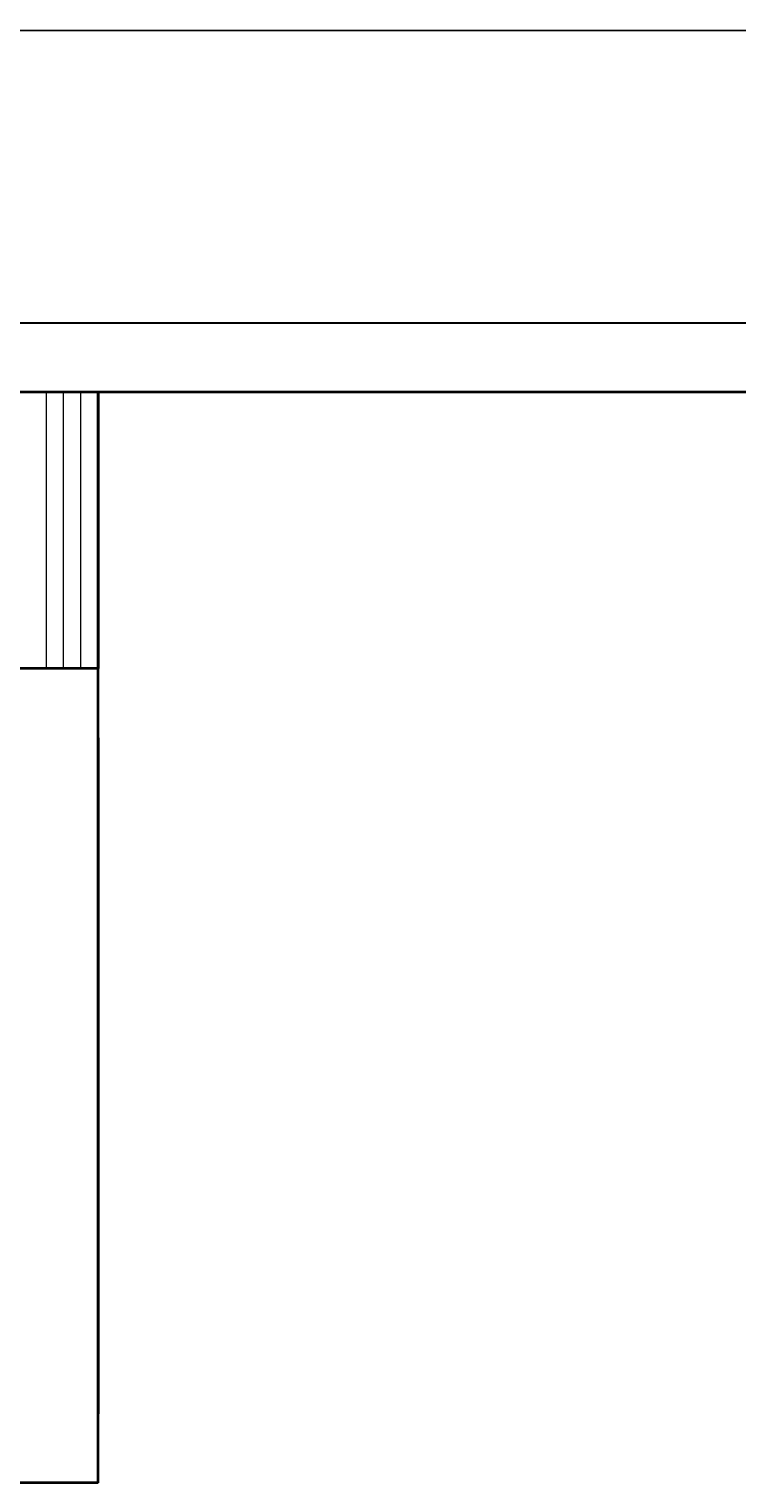
# Model space of a CAD drawing. Units: feet. Extents: x 2219 to 3039, y 1768 to 2369.
# Tile 7 of 16: x 2601 to 2694, y 2180 to 2369. Entities that reach past the tile are written whole.
import ezdxf

# ---------------------------------------------------------------- set-up
doc = ezdxf.new("R2010")
doc.units = ezdxf.units.FT
for name, color, linetype, lineweight in [('A-ANNO-DIMS', 2, 'Continuous', 18), ('A-FLOR-OPEN', 8, 'Continuous', 13), ('A-WALL', 7, 'Continuous', 35), ('C-PROP', 7, 'Continuous', 30)]:
    doc.layers.add(name, color=color, linetype=linetype, lineweight=lineweight)
doc.styles.get("Standard").update_dxf_attribs({"font": 'arial.ttf'})
doc.dimstyles.get("Standard").update_dxf_attribs({"dimtxt": 0.18, "dimasz": 0.18, "dimexe": 0.18, "dimexo": 0.0625, "dimgap": 0.09, "dimtad": 0, "dimtih": 1, "dimtoh": 1, "dimdec": 4, "dimzin": 0, "dimdsep": 46, "dimtxsty": 'Standard', "dimcen": 0.09, "dimadec": 0, "dimazin": 0, "dimtfac": 1, "dimtdec": 4, "dimtofl": 0, "dimtmove": 0, "dimatfit": 3, "dimfxl": 1, "dimtolj": 1, "dimtzin": 0, "dimarcsym": 0})

# ---------------------------------------------------------------- blocks, each defined once
blk = doc.blocks.new('*D55')
at = {"layer": 'A-ANNO-DIMS', "color": 0, "lineweight": -2, "transparency": 16777216}
for p, q in [((2400.38, 2330.99), (2400.38, 2369.15)), ((2400.56, 2368.97), (2561.1, 2368.97)), ((2722.22, 2368.97), (2561.68, 2368.97)), ((2722.4, 2330.99), (2722.4, 2369.15))]:
    blk.add_line(p, q, dxfattribs=at)
at = {"layer": 'A-ANNO-DIMS', "color": 0, "transparency": 16777216}
for points in [[(2400.56, 2369), (2400.56, 2368.94), (2400.38, 2368.97)], [(2722.22, 2369), (2722.22, 2368.94), (2722.4, 2368.97)]]:
    blk.add_solid(points, dxfattribs=at)
at = {"layer": 'Defpoints', "color": 0, "transparency": 16777216}
for p in [(2722.4, 2368.97), (2400.38, 2330.92), (2722.4, 2330.92)]:
    blk.add_point(p, dxfattribs=at)
at = {"layer": 'A-ANNO-DIMS', "color": 0, "transparency": 16777216, "insert": (2561.39, 2368.97), "char_height": 0.18, "attachment_point": 5}
blk.add_mtext('\\A1;322', dxfattribs=at)

msp = doc.modelspace()

# ---------------------------------------------------------------- linework, layer by layer
at = {"layer": 'A-FLOR-OPEN'}
for p, q in [((2603.65, 2285.923), (2603.65, 2321.923)), ((2605.9, 2285.923), (2605.9, 2321.923)), ((2608.15, 2285.923), (2608.15, 2321.923))]:
    msp.add_line(p, q, dxfattribs=at)
at = {"layer": 'A-WALL'}
for p, q in [((2532.4, 2321.923), (2610.4, 2321.923)), ((2610.4, 2321.923), (2610.4, 2285.923)), ((2610.4, 2321.923), (2834.4, 2321.923)), ((2610.4, 2179.923), (2610.4, 2321.923)), ((2610.4, 2285.923), (2532.4, 2285.923)), ((2610.4, 2276.923), (2610.4, 2188.923)), ((2610.4, 2179.923), (2532.4, 2179.923))]:
    msp.add_line(p, q, dxfattribs=at)
at = {"layer": 'C-PROP'}
msp.add_line((2314.4, 2330.923), (3000.4, 2330.923), dxfattribs=at)

# ---------------------------------------------------------------- dimensions: what is measured, and where the dimension line sits
at = {"layer": 'A-ANNO-DIMS'}
dim = msp.add_linear_dim(base=(2722.4, 2368.973), p1=(2400.382, 2330.923), p2=(2722.4, 2330.923), dimstyle='Standard', override={"dimdec": 0, "dimlfac": 1, "dimrnd": 0, "dimzin": 0, "dimdsep": 46, "dimlunit": 2}, dxfattribs=at)
dim.commit()
dim.dimension.update_dxf_attribs({"geometry": '*D55', "text_midpoint": (2561.391, 2368.973)})

doc.saveas('drawing.dxf')
